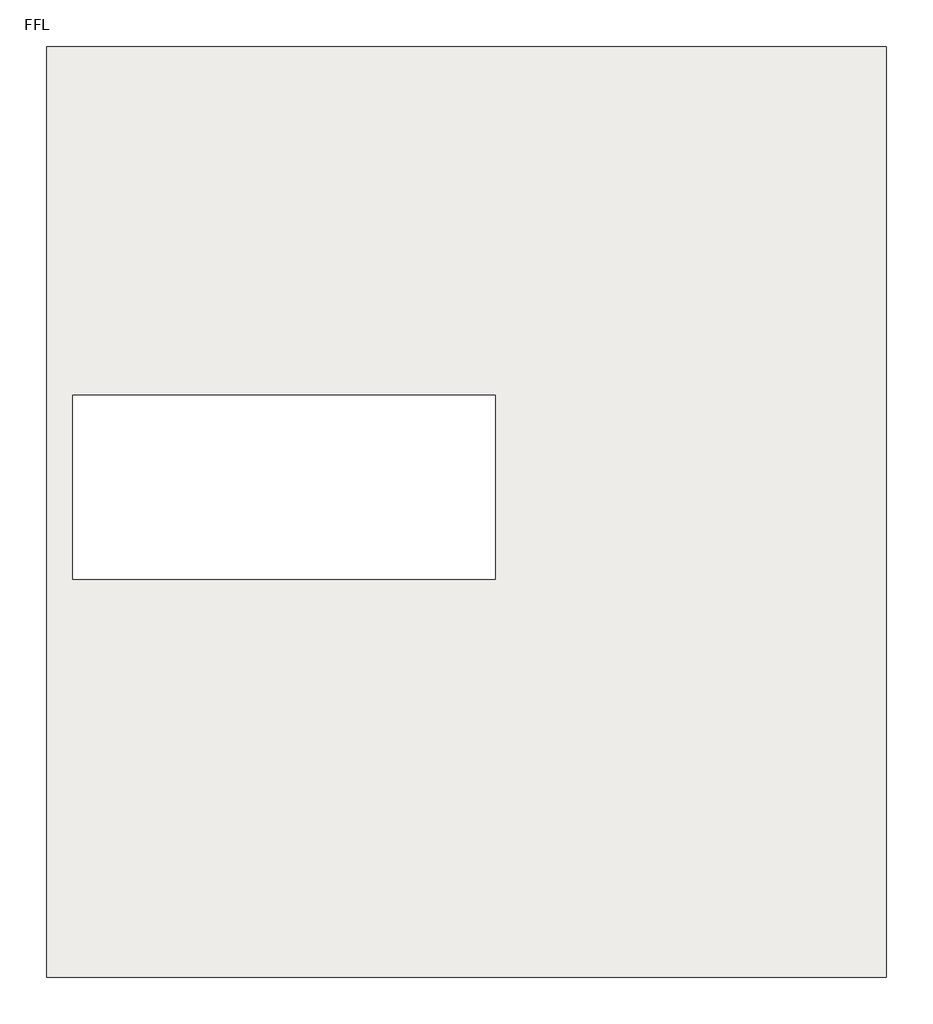
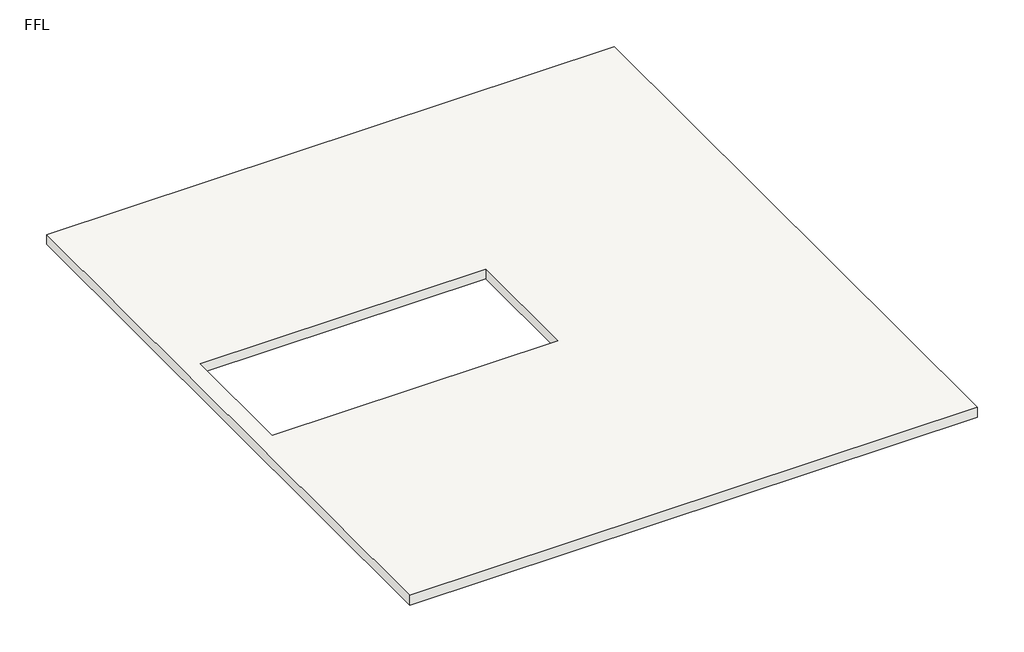
# One storey, incomplete: 1 slab.
"""IFC4 building model written with IfcOpenShell, lengths in millimetres."""

from ifc_helpers import new_model, si_unit, frame, origin, place, context, project, spatial, polyline, outline, extrude, element, save

model = new_model("IFC4")

# Units and contexts
model_context = context("Model", 3, world=origin())
ifc_project = project(units=[si_unit("LENGTHUNIT", "METRE", prefix="MILLI")], contexts=[model_context])

# Site, building, storey
site = spatial("IfcSite", under=ifc_project)
building = spatial("IfcBuilding", under=site)
storey = spatial("IfcBuildingStorey", under=building, Name="FFL", Elevation=3048.0)

# Slab
placement = place(None, origin())
element("IfcSlab", 1, ObjectType="SLAB", at=placement, inside=storey, context=model_context, shape_type="SweptSolid", body=[
    extrude(outline(polyline([(-3051.0504231, 10849.7806314), (-3051.0504231, 1705.7806314), (-11298.4304231, 1705.7806314), (-11298.4304231, 10849.7806314), (-3051.0504231, 10849.7806314)]), holes=[polyline([(-6892.1428068, 7426.4671174), (-11039.3504231, 7426.4671174), (-11039.3504231, 5614.7791611), (-6892.1428068, 5614.7791611), (-6892.1428068, 7426.4671174)])]), frame((0.0, 0.0, 3048.0), z_axis=(0.0, 0.0, 1.0), x_axis=(1.0, 0.0, 0.0)), (0.0, 0.0, 1.0), 149.9616),
])

save(model, "model.ifc")

# Revit data of these elements
# Type "SLAB"
#   Layers, outside or top first: 0.492 ft "Concrete, Precast" (function 1)
# Element 1 (IfcSlab, "SLAB")
#   Height Offset From Level = 0.492 ft
#   built-in parameter 1001954 = 1
#   Phase Created = New Construction
#   Materials on its faces: "Concrete, Precast"
# Materials
#   "Concrete, Precast": class "Concrete", colour RGB 192 192 192, transparency 0, Description = "Precast concrete", Cost = 0
